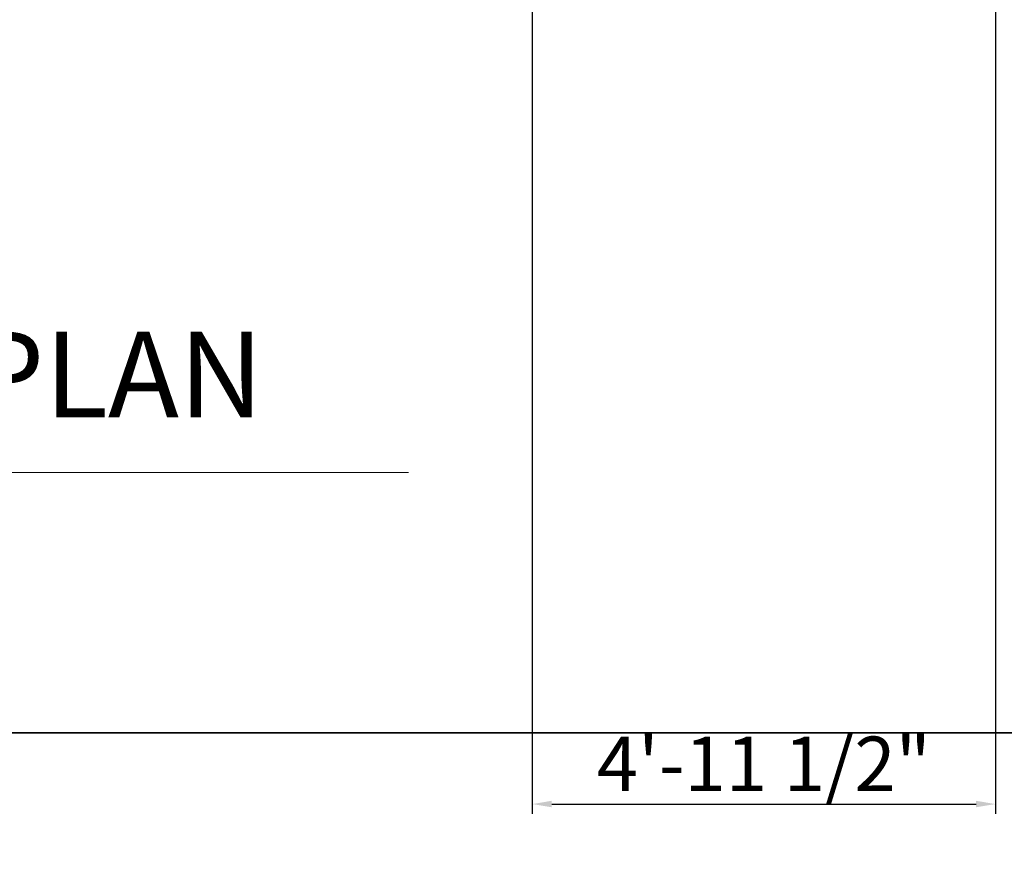
# Model space of a CAD drawing. Units: inches. Extents: x 1863 to 2938, y 1238 to 2492.
# Tile 2 of 12: x 2158 to 2285, y 1238 to 1345. Entities that reach past the tile are written whole.
import ezdxf

# ---------------------------------------------------------------- set-up
doc = ezdxf.new("R2010")
doc.units = ezdxf.units.IN
for name, color, linetype, lineweight in [('A-ANNO-DIMS', 2, 'Continuous', 18), ('A-ANNO-TEXT', 7, 'Continuous', 18), ('A-ANNO-TTLB', 7, 'Continuous', 35)]:
    doc.layers.add(name, color=color, linetype=linetype, lineweight=lineweight)
doc.styles.get("Standard").update_dxf_attribs({"font": 'arial.ttf'})
doc.dimstyles.new('ISO-25', dxfattribs={"dimtxt": 7, "dimasz": 2.5, "dimexe": 1.25, "dimexo": 0.625, "dimtad": 1, "dimdec": 0, "dimlunit": 3, "dimtxsty": 'Standard', "dimcen": 2.5, "dimadec": 0, "dimazin": 0, "dimtfac": 1, "dimtdec": 0, "dimtmove": 0, "dimatfit": 3, "dimfxl": 1, "dimarcsym": 0})

# ---------------------------------------------------------------- blocks, each defined once
blk = doc.blocks.new('*D58')
at = {"layer": 'A-ANNO-DIMS', "color": 0, "lineweight": -2, "transparency": 16777216}
for p, q in [((2283.38, 1624.45), (2283.38, 1243.07)), ((2223.92, 1623.6), (2223.92, 1243.07)), ((2226.42, 1244.32), (2280.88, 1244.32))]:
    blk.add_line(p, q, dxfattribs=at)
at = {"layer": 'A-ANNO-DIMS', "color": 0, "transparency": 16777216}
for points in [[(2226.42, 1244.74), (2226.42, 1243.91), (2223.92, 1244.32)], [(2280.88, 1244.74), (2280.88, 1243.91), (2283.38, 1244.32)]]:
    blk.add_solid(points, dxfattribs=at)
at = {"layer": 'Defpoints', "color": 0, "transparency": 16777216}
for p in [(2223.92, 1624.22), (2283.38, 1625.07), (2283.38, 1244.32)]:
    blk.add_point(p, dxfattribs=at)
at = {"layer": 'A-ANNO-DIMS', "color": 0, "transparency": 16777216, "insert": (2253.65, 1248.57), "char_height": 7, "attachment_point": 5}
blk.add_mtext('4\'-11 1/2"', dxfattribs=at)

msp = doc.modelspace()

# ---------------------------------------------------------------- linework, layer by layer
at = {"layer": 'A-ANNO-TEXT'}
msp.add_line((2031.3, 1286.87), (2208.05, 1286.87), dxfattribs=at)
at = {"layer": 'A-ANNO-TTLB'}
msp.add_lwpolyline([(1863.2, 2492.19), (2938.41, 2492.19), (2938.41, 1253.47), (1863.2, 1253.47)], close=True, dxfattribs=at)

# ---------------------------------------------------------------- texts
at = {"layer": 'A-ANNO-TEXT', "insert": (2033.86, 1304.94), "char_height": 11, "attachment_point": 1}
msp.add_mtext_dynamic_manual_height_columns('GROUND FLOOR PLAN', width=285.9914, gutter_width=12.5, heights=[0], dxfattribs=at)

# ---------------------------------------------------------------- dimensions: what is measured, and where the dimension line sits
at = {"layer": 'A-ANNO-DIMS'}
dim = msp.add_linear_dim(base=(2283.38, 1244.32), p1=(2223.92, 1624.22), p2=(2283.38, 1625.07), dimstyle='ISO-25', override={"dimdec": 1, "dimlfac": 1, "dimrnd": 0, "dimzin": 1, "dimdsep": 46, "dimlunit": 4, "dimfrac": 2}, dxfattribs=at)
dim.commit()
dim.dimension.update_dxf_attribs({"geometry": '*D58', "text_midpoint": (2253.65, 1248.57)})

doc.saveas('drawing.dxf')
